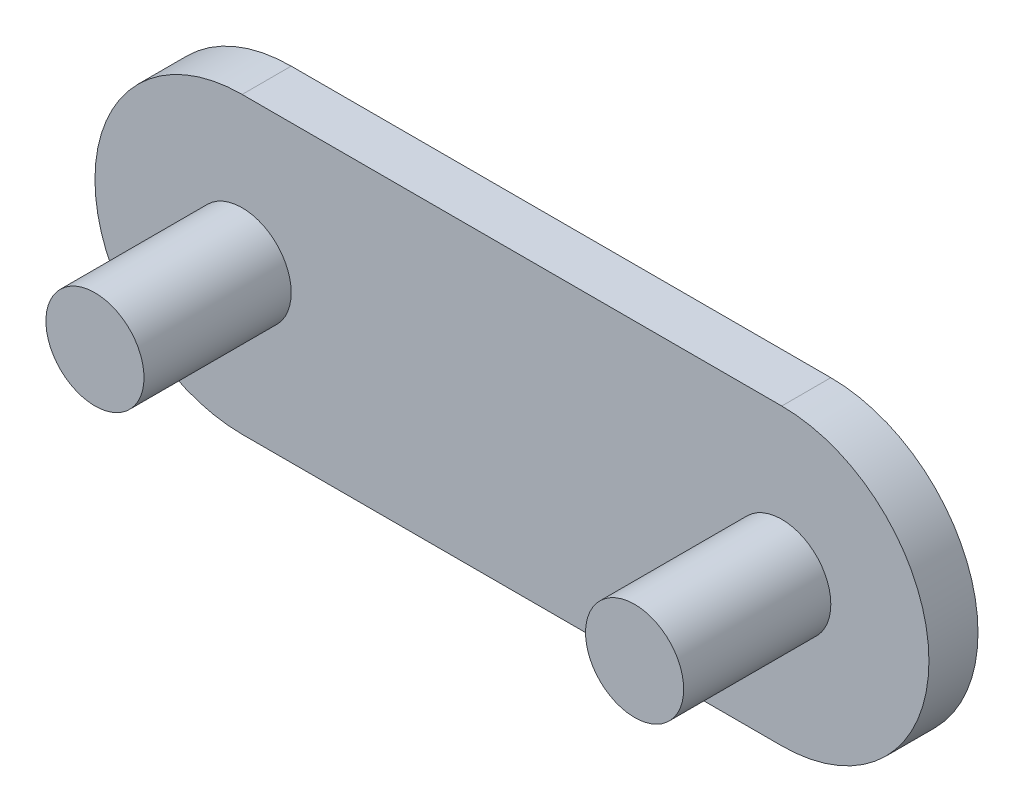
ISO-10303-21;
HEADER;
FILE_DESCRIPTION(('STEP AP214'),'2;1');
FILE_NAME('part.step','',(''),(''),'','','');
FILE_SCHEMA(('AUTOMOTIVE_DESIGN { 1 0 10303 214 1 1 1 1 }'));
ENDSEC;
DATA;
#1=APPLICATION_CONTEXT('core data for automotive mechanical design processes');
#2=APPLICATION_PROTOCOL_DEFINITION('international standard','automotive_design',2000,#1);
#3=PRODUCT_CONTEXT('',#1,'mechanical');
#4=PRODUCT('Part','Part','',(#3));
#5=PRODUCT_RELATED_PRODUCT_CATEGORY('part','',(#4));
#6=PRODUCT_DEFINITION_FORMATION('','',#4);
#7=PRODUCT_DEFINITION_CONTEXT('part definition',#1,'design');
#8=PRODUCT_DEFINITION('design','',#6,#7);
#9=PRODUCT_DEFINITION_SHAPE('','',#8);
#10=(LENGTH_UNIT() NAMED_UNIT(*) SI_UNIT(.MILLI.,.METRE.));
#11=(NAMED_UNIT(*) PLANE_ANGLE_UNIT() SI_UNIT($,.RADIAN.));
#12=(NAMED_UNIT(*) SI_UNIT($,.STERADIAN.) SOLID_ANGLE_UNIT());
#13=UNCERTAINTY_MEASURE_WITH_UNIT(LENGTH_MEASURE(1.E-05),#10,'distance_accuracy_value','');
#14=(GEOMETRIC_REPRESENTATION_CONTEXT(3) GLOBAL_UNCERTAINTY_ASSIGNED_CONTEXT((#13)) GLOBAL_UNIT_ASSIGNED_CONTEXT((#10,
#11,#12)) REPRESENTATION_CONTEXT('',''));
#15=CARTESIAN_POINT('',(0.,0.,0.));
#16=DIRECTION('',(0.,0.,1.));
#17=DIRECTION('',(1.,0.,0.));
#18=AXIS2_PLACEMENT_3D('',#15,#16,#17);
#19=CARTESIAN_POINT('',(-27.5,0.,5.));
#20=DIRECTION('',(0.,0.,-1.));
#21=DIRECTION('',(-1.,0.,0.));
#22=AXIS2_PLACEMENT_3D('',#19,#20,#21);
#23=CYLINDRICAL_SURFACE('',#22,15.);
#24=CARTESIAN_POINT('',(-27.5,0.,0.));
#25=DIRECTION('',(0.,0.,1.));
#26=DIRECTION('',(1.,0.,0.));
#27=AXIS2_PLACEMENT_3D('',#24,#25,#26);
#28=CIRCLE('',#27,15.);
#29=CARTESIAN_POINT('',(-27.5,15.,0.));
#30=VERTEX_POINT('',#29);
#31=CARTESIAN_POINT('',(-27.5,-15.,0.));
#32=VERTEX_POINT('',#31);
#33=EDGE_CURVE('E105',#30,#32,#28,.T.);
#34=ORIENTED_EDGE('',*,*,#33,.T.);
#35=DIRECTION('',(0.,0.,-1.));
#36=VECTOR('',#35,1.);
#37=CARTESIAN_POINT('',(-27.5,-15.,5.));
#38=LINE('',#37,#36);
#39=CARTESIAN_POINT('',(-27.5,-15.,5.));
#40=VERTEX_POINT('',#39);
#41=EDGE_CURVE('E11',#40,#32,#38,.T.);
#42=ORIENTED_EDGE('',*,*,#41,.F.);
#43=CARTESIAN_POINT('',(-27.5,0.,5.));
#44=DIRECTION('',(0.,0.,1.));
#45=DIRECTION('',(1.,0.,0.));
#46=AXIS2_PLACEMENT_3D('',#43,#44,#45);
#47=CIRCLE('',#46,15.);
#48=CARTESIAN_POINT('',(-27.5,15.,5.));
#49=VERTEX_POINT('',#48);
#50=EDGE_CURVE('E89',#49,#40,#47,.T.);
#51=ORIENTED_EDGE('',*,*,#50,.F.);
#52=DIRECTION('',(0.,0.,-1.));
#53=VECTOR('',#52,1.);
#54=CARTESIAN_POINT('',(-27.5,15.,5.));
#55=LINE('',#54,#53);
#56=EDGE_CURVE('E98',#49,#30,#55,.T.);
#57=ORIENTED_EDGE('',*,*,#56,.T.);
#58=EDGE_LOOP('',(#34,#42,#51,#57));
#59=FACE_BOUND('',#58,.T.);
#60=ADVANCED_FACE('F39',(#59),#23,.T.);
#61=CARTESIAN_POINT('',(-27.5,-15.,5.));
#62=DIRECTION('',(0.,1.,0.));
#63=DIRECTION('',(-1.,0.,0.));
#64=AXIS2_PLACEMENT_3D('',#61,#62,#63);
#65=PLANE('',#64);
#66=DIRECTION('',(1.,0.,0.));
#67=VECTOR('',#66,1.);
#68=CARTESIAN_POINT('',(-27.5,-15.,0.));
#69=LINE('',#68,#67);
#70=CARTESIAN_POINT('',(27.5,-15.,0.));
#71=VERTEX_POINT('',#70);
#72=EDGE_CURVE('E94',#32,#71,#69,.T.);
#73=ORIENTED_EDGE('',*,*,#72,.T.);
#74=DIRECTION('',(0.,0.,-1.));
#75=VECTOR('',#74,1.);
#76=CARTESIAN_POINT('',(27.5,-15.,5.));
#77=LINE('',#76,#75);
#78=CARTESIAN_POINT('',(27.5,-15.,5.));
#79=VERTEX_POINT('',#78);
#80=EDGE_CURVE('E50',#79,#71,#77,.T.);
#81=ORIENTED_EDGE('',*,*,#80,.F.);
#82=DIRECTION('',(1.,0.,0.));
#83=VECTOR('',#82,1.);
#84=CARTESIAN_POINT('',(-27.5,-15.,5.));
#85=LINE('',#84,#83);
#86=EDGE_CURVE('E81',#40,#79,#85,.T.);
#87=ORIENTED_EDGE('',*,*,#86,.F.);
#88=ORIENTED_EDGE('',*,*,#41,.T.);
#89=EDGE_LOOP('',(#73,#81,#87,#88));
#90=FACE_BOUND('',#89,.T.);
#91=ADVANCED_FACE('F91',(#90),#65,.F.);
#92=CARTESIAN_POINT('',(27.5,0.,5.));
#93=DIRECTION('',(0.,0.,-1.));
#94=DIRECTION('',(-1.,0.,0.));
#95=AXIS2_PLACEMENT_3D('',#92,#93,#94);
#96=CYLINDRICAL_SURFACE('',#95,15.);
#97=CARTESIAN_POINT('',(27.5,0.,0.));
#98=DIRECTION('',(0.,0.,1.));
#99=DIRECTION('',(1.,0.,0.));
#100=AXIS2_PLACEMENT_3D('',#97,#98,#99);
#101=CIRCLE('',#100,15.);
#102=CARTESIAN_POINT('',(27.5,15.,0.));
#103=VERTEX_POINT('',#102);
#104=EDGE_CURVE('E75',#71,#103,#101,.T.);
#105=ORIENTED_EDGE('',*,*,#104,.T.);
#106=DIRECTION('',(0.,0.,-1.));
#107=VECTOR('',#106,1.);
#108=CARTESIAN_POINT('',(27.5,15.,5.));
#109=LINE('',#108,#107);
#110=CARTESIAN_POINT('',(27.5,15.,5.));
#111=VERTEX_POINT('',#110);
#112=EDGE_CURVE('E92',#111,#103,#109,.T.);
#113=ORIENTED_EDGE('',*,*,#112,.F.);
#114=CARTESIAN_POINT('',(27.5,0.,5.));
#115=DIRECTION('',(0.,0.,1.));
#116=DIRECTION('',(1.,0.,0.));
#117=AXIS2_PLACEMENT_3D('',#114,#115,#116);
#118=CIRCLE('',#117,15.);
#119=EDGE_CURVE('E86',#79,#111,#118,.T.);
#120=ORIENTED_EDGE('',*,*,#119,.F.);
#121=ORIENTED_EDGE('',*,*,#80,.T.);
#122=EDGE_LOOP('',(#105,#113,#120,#121));
#123=FACE_BOUND('',#122,.T.);
#124=ADVANCED_FACE('F96',(#123),#96,.T.);
#125=CARTESIAN_POINT('',(-27.5,15.,5.));
#126=DIRECTION('',(0.,-1.,0.));
#127=DIRECTION('',(1.,0.,0.));
#128=AXIS2_PLACEMENT_3D('',#125,#126,#127);
#129=PLANE('',#128);
#130=DIRECTION('',(-1.,0.,0.));
#131=VECTOR('',#130,1.);
#132=CARTESIAN_POINT('',(-27.5,15.,0.));
#133=LINE('',#132,#131);
#134=EDGE_CURVE('E80',#103,#30,#133,.T.);
#135=ORIENTED_EDGE('',*,*,#134,.T.);
#136=ORIENTED_EDGE('',*,*,#56,.F.);
#137=DIRECTION('',(-1.,0.,0.));
#138=VECTOR('',#137,1.);
#139=CARTESIAN_POINT('',(-27.5,15.,5.));
#140=LINE('',#139,#138);
#141=EDGE_CURVE('E54',#111,#49,#140,.T.);
#142=ORIENTED_EDGE('',*,*,#141,.F.);
#143=ORIENTED_EDGE('',*,*,#112,.T.);
#144=EDGE_LOOP('',(#135,#136,#142,#143));
#145=FACE_BOUND('',#144,.T.);
#146=ADVANCED_FACE('F109',(#145),#129,.F.);
#147=CARTESIAN_POINT('',(-27.5,0.,5.));
#148=DIRECTION('',(0.,0.,1.));
#149=DIRECTION('',(1.,0.,0.));
#150=AXIS2_PLACEMENT_3D('',#147,#148,#149);
#151=PLANE('',#150);
#152=CARTESIAN_POINT('',(27.5,0.,5.));
#153=DIRECTION('',(0.,0.,1.));
#154=DIRECTION('',(1.,0.,0.));
#155=AXIS2_PLACEMENT_3D('',#152,#153,#154);
#156=CIRCLE('',#155,5.);
#157=CARTESIAN_POINT('',(32.5,0.,5.));
#158=VERTEX_POINT('',#157);
#159=EDGE_CURVE('E125',#158,#158,#156,.T.);
#160=ORIENTED_EDGE('',*,*,#159,.F.);
#161=EDGE_LOOP('',(#160));
#162=FACE_BOUND('',#161,.T.);
#163=CARTESIAN_POINT('',(-27.5,0.,5.));
#164=DIRECTION('',(0.,0.,1.));
#165=DIRECTION('',(1.,0.,0.));
#166=AXIS2_PLACEMENT_3D('',#163,#164,#165);
#167=CIRCLE('',#166,5.);
#168=CARTESIAN_POINT('',(-22.5,0.,5.));
#169=VERTEX_POINT('',#168);
#170=EDGE_CURVE('E119',#169,#169,#167,.T.);
#171=ORIENTED_EDGE('',*,*,#170,.F.);
#172=EDGE_LOOP('',(#171));
#173=FACE_BOUND('',#172,.T.);
#174=ORIENTED_EDGE('',*,*,#50,.T.);
#175=ORIENTED_EDGE('',*,*,#86,.T.);
#176=ORIENTED_EDGE('',*,*,#119,.T.);
#177=ORIENTED_EDGE('',*,*,#141,.T.);
#178=EDGE_LOOP('',(#174,#175,#176,#177));
#179=FACE_BOUND('',#178,.T.);
#180=ADVANCED_FACE('F88',(#162,#173,#179),#151,.T.);
#181=CARTESIAN_POINT('',(-27.5,0.,0.));
#182=DIRECTION('',(0.,0.,1.));
#183=DIRECTION('',(1.,0.,0.));
#184=AXIS2_PLACEMENT_3D('',#181,#182,#183);
#185=PLANE('',#184);
#186=ORIENTED_EDGE('',*,*,#33,.F.);
#187=ORIENTED_EDGE('',*,*,#134,.F.);
#188=ORIENTED_EDGE('',*,*,#104,.F.);
#189=ORIENTED_EDGE('',*,*,#72,.F.);
#190=EDGE_LOOP('',(#186,#187,#188,#189));
#191=FACE_BOUND('',#190,.T.);
#192=ADVANCED_FACE('F114',(#191),#185,.F.);
#193=CARTESIAN_POINT('',(-27.5,0.,20.));
#194=DIRECTION('',(0.,0.,-1.));
#195=DIRECTION('',(-1.,0.,0.));
#196=AXIS2_PLACEMENT_3D('',#193,#194,#195);
#197=CYLINDRICAL_SURFACE('',#196,5.);
#198=CARTESIAN_POINT('',(-27.5,0.,20.));
#199=DIRECTION('',(0.,0.,1.));
#200=DIRECTION('',(1.,0.,0.));
#201=AXIS2_PLACEMENT_3D('',#198,#199,#200);
#202=CIRCLE('',#201,5.);
#203=CARTESIAN_POINT('',(-22.5,0.,20.));
#204=VERTEX_POINT('',#203);
#205=EDGE_CURVE('E104',#204,#204,#202,.T.);
#206=ORIENTED_EDGE('',*,*,#205,.F.);
#207=EDGE_LOOP('',(#206));
#208=FACE_BOUND('',#207,.T.);
#209=ORIENTED_EDGE('',*,*,#170,.T.);
#210=EDGE_LOOP('',(#209));
#211=FACE_BOUND('',#210,.T.);
#212=ADVANCED_FACE('F142',(#208,#211),#197,.T.);
#213=CARTESIAN_POINT('',(-27.5,0.,20.));
#214=DIRECTION('',(0.,0.,1.));
#215=DIRECTION('',(1.,0.,0.));
#216=AXIS2_PLACEMENT_3D('',#213,#214,#215);
#217=PLANE('',#216);
#218=ORIENTED_EDGE('',*,*,#205,.T.);
#219=EDGE_LOOP('',(#218));
#220=FACE_BOUND('',#219,.T.);
#221=ADVANCED_FACE('F135',(#220),#217,.T.);
#222=CARTESIAN_POINT('',(27.5,0.,20.));
#223=DIRECTION('',(0.,0.,-1.));
#224=DIRECTION('',(-1.,0.,0.));
#225=AXIS2_PLACEMENT_3D('',#222,#223,#224);
#226=CYLINDRICAL_SURFACE('',#225,5.);
#227=CARTESIAN_POINT('',(27.5,0.,20.));
#228=DIRECTION('',(0.,0.,1.));
#229=DIRECTION('',(1.,0.,0.));
#230=AXIS2_PLACEMENT_3D('',#227,#228,#229);
#231=CIRCLE('',#230,5.);
#232=CARTESIAN_POINT('',(32.5,0.,20.));
#233=VERTEX_POINT('',#232);
#234=EDGE_CURVE('E118',#233,#233,#231,.T.);
#235=ORIENTED_EDGE('',*,*,#234,.F.);
#236=EDGE_LOOP('',(#235));
#237=FACE_BOUND('',#236,.T.);
#238=ORIENTED_EDGE('',*,*,#159,.T.);
#239=EDGE_LOOP('',(#238));
#240=FACE_BOUND('',#239,.T.);
#241=ADVANCED_FACE('F128',(#237,#240),#226,.T.);
#242=CARTESIAN_POINT('',(27.5,0.,20.));
#243=DIRECTION('',(0.,0.,1.));
#244=DIRECTION('',(1.,0.,0.));
#245=AXIS2_PLACEMENT_3D('',#242,#243,#244);
#246=PLANE('',#245);
#247=ORIENTED_EDGE('',*,*,#234,.T.);
#248=EDGE_LOOP('',(#247));
#249=FACE_BOUND('',#248,.T.);
#250=ADVANCED_FACE('F126',(#249),#246,.T.);
#251=CLOSED_SHELL('',(#60,#91,#124,#146,#180,#192,#212,#221,#241,#250));
#252=MANIFOLD_SOLID_BREP('B2',#251);
#253=ADVANCED_BREP_SHAPE_REPRESENTATION('',(#18,#252),#14);
#254=SHAPE_DEFINITION_REPRESENTATION(#9,#253);
ENDSEC;
END-ISO-10303-21;
